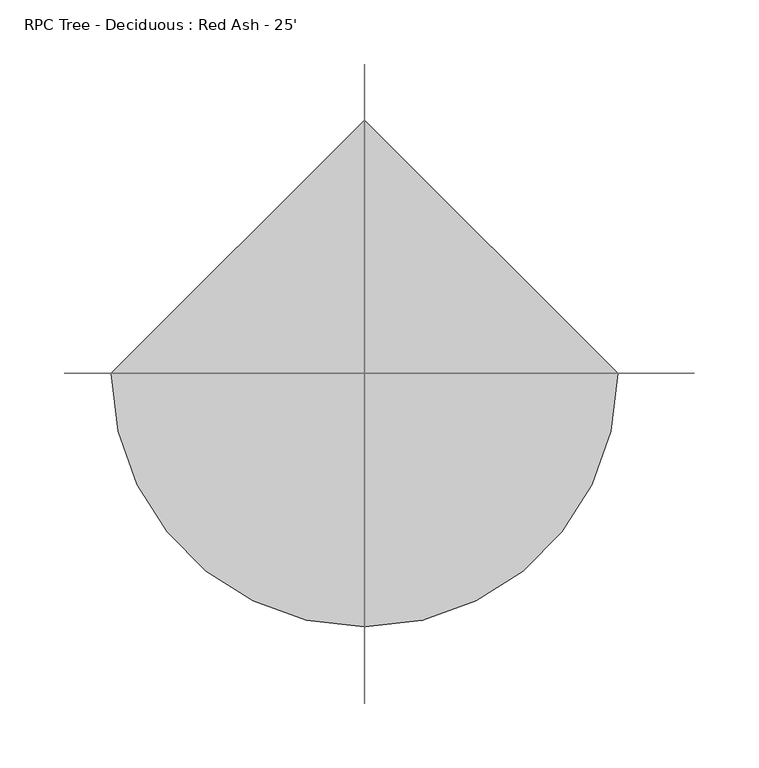
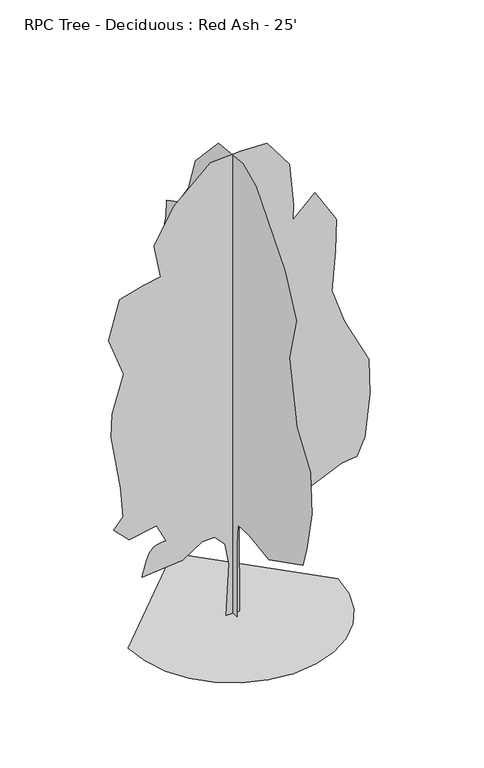
"""IFC4 building model written with IfcOpenShell, lengths in millimetres: geographic element geometry, RPC Tree - Deciduous : Red Ash - 25'."""

from ifc_helpers import new_model, si_unit, origin, place, context, project, spatial, triangles, source, transform, mapped, element, save


def rpc_tree_deciduous_red_ash_25_29d6c0be(model_context):
    return source(origin(), model_context, "Body", "Tessellation", [
        triangles([(-197.3943103, 0.0, 7.4e-06), (-192.1758061, -45.2297202, 7.4e-06), (-177.3137228, -86.7659884, 7.4e-06), (-153.9979766, -123.4187294, 7.4e-06), (-123.4187385, -153.9979948, 7.4e-06), (-86.7659612, -177.3136864, 7.4e-06), (-45.229702, -192.1758061, 7.4e-06), (8.6e-06, -197.3943103, 7.4e-06), (45.2297247, -192.1758243, 7.4e-06), (86.7659884, -177.3137228, 7.4e-06), (123.4187385, -153.9979766, 7.4e-06), (153.9980311, -123.4187385, 7.4e-06), (177.3137046, -86.7659612, 7.4e-06), (192.1758061, -45.2296929, 7.4e-06), (197.3943103, 1.73e-05, 7.4e-06), (-2.59e-05, 197.3943103, 7.4e-06), (-1.3e-06, -12.3415511, 0.0), (3e-06, -12.1496059, 143.3464828), (3.9e-06, -15.5858355, 184.536356), (1e-07, -52.659045, 186.979866), (-6.9e-06, -117.166958, 177.3968209), (-1.69e-05, -228.4431237, 233.8412498), (-1.7e-05, -241.3447163, 275.7714303), (-1.63e-05, -257.4717115, 353.1809132), (-1.34e-05, -252.6336529, 433.8158532), (-7e-06, -208.845846, 496.9220667), (-7e-07, -183.2878312, 619.2762262), (-4e-07, -205.8654139, 706.361899), (5.8e-06, -168.773401, 783.7714182), (1.88e-05, -75.2369229, 895.0476202), (2.38e-05, -32.784084, 914.1832981), (3.19e-05, 47.3281931, 906.3365387), (3.75e-05, 123.1250246, 825.701635), (3.78e-05, 145.7028252, 757.9682693), (3.99e-05, 179.5693627, 709.5872835), (4.32e-05, 216.6615754, 690.2349764), (4.24e-05, 218.2742676, 657.9809132), (4.23e-05, 227.9504757, 620.8889185), (3.93e-05, 211.8234986, 577.3460458), (3.96e-05, 226.3377653, 535.4159017), (3.93e-05, 240.8520501, 477.3587623), (3.85e-05, 237.6266656, 461.2317307), (3.45e-05, 210.2108063, 422.5269711), (3.28e-05, 208.4773911, 369.3079448), (3.16e-05, 206.9853855, 335.441262), (3.05e-05, 208.5980959, 293.511136), (2.89e-05, 210.2108245, 235.4540148), (2.61e-05, 187.6330238, 217.7142909), (2.17e-05, 145.7028797, 217.7142909), (2.19e-05, 165.0552595, 158.0444592), (2.06e-05, 161.8194105, 124.1861426), (1.82e-05, 132.363723, 147.3403706), (1.18e-05, 75.5355238, 132.8049115), (1.18e-05, 66.2054202, 162.8473093), (7.5e-06, 25.9095309, 162.4803077), (6e-06, 15.6961474, 147.4001417), (3.9e-06, 9.5459199, 98.1939791), (1.4e-06, 13.4599217, 1.5e-06), (-13.3045045, 6e-07, 5.4e-06), (-8.005377, -1.16e-05, 100.020203), (-15.5168751, -1.63e-05, 142.5532264), (-34.8945452, -1.8e-05, 163.8381281), (-58.0363739, -1.69e-05, 163.0435545), (-95.5521345, -1.24e-05, 138.6920794), (-171.3489706, -8.3e-06, 132.2413013), (-170.3004699, -8.8e-06, 136.411759), (-169.1814611, -9.4e-06, 140.72326), (-167.9214, -1e-05, 145.3168386), (-166.4497602, -1.06e-05, 150.3336381), (-164.6960155, -1.14e-05, 155.9145202), (-162.5896397, -1.22e-05, 162.2008008), (-160.0601066, -1.32e-05, 169.3333414), (-156.8723288, -1.41e-05, 175.948708), (-152.9228605, -1.49e-05, 180.7868029), (-148.3386563, -1.55e-05, 184.1437928), (-143.2466434, -1.59e-05, 186.3160621), (-137.7738306, -1.63e-05, 187.5995956), (-132.0470817, -1.67e-05, 188.2907417), (-126.1933965, -1.7e-05, 188.6857212), (-143.9330659, -2.04e-05, 224.1650781), (-195.5394453, -1.7e-05, 214.4888882), (-224.5679605, -1.92e-05, 243.5175124), (-206.8282911, -2.25e-05, 264.4825845), (-211.6663679, -2.92e-05, 322.5397239), (-229.4060555, -4.13e-05, 430.5904687), (-227.8176895, -4.67e-05, 475.3398448), (-206.3900911, -5.63e-05, 547.5990606), (-234.2441686, -6.42e-05, 624.1142303), (-213.279042, -7.39e-05, 698.2984377), (-169.736242, -7.74e-05, 711.1999758), (-136.6095848, -7.95e-05, 717.0435144), (-148.7711881, -8.67e-05, 782.1587259), (-111.6790935, -9.62e-05, 848.2793993), (-42.3330356, -0.0001068, 911.1746155), (14.1113616, -0.0001096, 914.4), (64.1050488, -0.0001116, 912.7872351), (106.0352065, -0.0001067, 856.3428606), (113.7446469, -9.72e-05, 773.7021927), (112.6376287, -9.35e-05, 743.396339), (154.4161378, -0.0001, 782.1587259), (194.7336079, -9.39e-05, 716.0380526), (193.1209156, -8.64e-05, 653.5811817), (185.9348898, -7.68e-05, 576.0782453), (209.2478927, -6.97e-05, 507.9999879), (255.811693, -6.08e-05, 416.3037681), (257.2962499, -5.26e-05, 347.1371324), (247.9526341, -4.24e-05, 264.4825481), (233.4383493, -3.77e-05, 230.6158653), (204.4097796, -3.6e-05, 227.3904808), (147.9653506, -3.05e-05, 201.5872956), (97.9716635, -2.41e-05, 166.1079387), (30.8971852, -2.46e-05, 194.9482568), (11.166104, -2.12e-05, 173.7161771), (12.4986284, -5e-07, 4.2e-06)], [[15, 16, 1], [14, 15, 1], [14, 1, 2], [13, 14, 2], [13, 2, 3], [13, 3, 4], [12, 13, 4], [11, 12, 4], [11, 4, 5], [11, 5, 6], [11, 6, 7], [11, 7, 8], [11, 8, 9], [11, 9, 10], [50, 51, 52], [57, 58, 17], [57, 17, 18], [56, 57, 18], [56, 18, 19], [55, 56, 19], [49, 50, 52], [52, 53, 54], [49, 52, 54], [35, 36, 37], [46, 47, 48], [46, 48, 49], [21, 22, 23], [20, 21, 23], [20, 23, 24], [20, 24, 25], [20, 25, 26], [19, 20, 26], [19, 26, 27], [45, 46, 49], [31, 32, 33], [30, 31, 33], [29, 30, 33], [29, 33, 34], [28, 29, 34], [27, 28, 34], [19, 27, 34], [19, 34, 35], [19, 35, 37], [19, 37, 38], [19, 38, 39], [19, 39, 40], [19, 40, 41], [19, 41, 42], [19, 42, 43], [19, 43, 44], [19, 44, 45], [19, 45, 49], [19, 49, 54], [55, 19, 54], [64, 65, 66], [64, 66, 67], [64, 67, 68], [99, 100, 101], [64, 68, 69], [64, 69, 70], [64, 70, 71], [114, 59, 60], [113, 114, 60], [113, 60, 61], [113, 61, 62], [64, 71, 72], [64, 72, 73], [64, 73, 74], [64, 74, 75], [64, 75, 76], [64, 76, 77], [64, 77, 78], [64, 78, 79], [63, 64, 79], [81, 82, 83], [80, 81, 83], [99, 101, 102], [107, 108, 109], [110, 111, 112], [88, 89, 90], [87, 88, 90], [87, 90, 91], [80, 83, 84], [95, 96, 97], [95, 97, 98], [94, 95, 98], [93, 94, 98], [92, 93, 98], [91, 92, 98], [91, 98, 99], [87, 91, 99], [87, 99, 102], [87, 102, 103], [87, 103, 104], [86, 87, 104], [85, 86, 104], [84, 85, 104], [80, 84, 104], [80, 104, 105], [80, 105, 106], [80, 106, 107], [80, 107, 109], [80, 109, 110], [80, 110, 112], [79, 80, 112], [63, 79, 112], [62, 63, 112], [113, 62, 112]], closed=False),
    ])


if __name__ == "__main__":
    model = new_model("IFC4")
    model_context = context("Model", 3, world=origin())
    ifc_project = project(units=[si_unit("LENGTHUNIT", "METRE", prefix="MILLI")], contexts=[model_context])
    site = spatial("IfcSite", under=ifc_project)
    building = spatial("IfcBuilding", under=site)
    placement = place(None, origin())
    rpc_tree_deciduous_red_ash_25_shape = rpc_tree_deciduous_red_ash_25_29d6c0be(model_context)
    element("IfcGeographicElement", 1, ObjectType="RPC Tree - Deciduous : Red Ash - 25'", at=placement, inside=building, context=model_context, shape_type="MappedRepresentation", body=[
        mapped(rpc_tree_deciduous_red_ash_25_shape, transform((0.0, 0.0, 0.0), x_axis=(1.0, 0.0, 0.0), y_axis=(0.0, 1.0, 0.0), z_axis=(0.0, 0.0, 1.0))),
    ])
    save(model, "model.ifc")

# Revit data of these elements
# Type "RPC Tree - Deciduous : Red Ash - 25'"
#   built-in parameter 1005198 = "{2, 15},{22, RPC-8-G3GR-497X-PHW5-6},{1, 0},{1, 0},{2, 15},{1, 8},{5, Color},{1, 0},{1, 0},{3, 0.8},{3, 0.8},{3, 0.8},{1, 8},{7, BBoxMin},{1, 0},{1, 0},{1, 0},{1, 0},{1, 0},{1, 8},{7, BBoxMax},{1, 0},{1, 0},{1, 0},{1, 0},{1, 0},{2, 11},{9, RPCTypeId},{1, 0},{1, 0},{22, RPC-8-G3GR-497X-PHW5-6},{1, 6},{14, RPCPlantHeight},{1, 0},{1, 0},{2, 25},{2, 11},{7, keyword},{1, 0},{1, 0},{34, :RPCs:Trees [General]:Geometry:RPC},{2, 11},{8, category},{1, 0},{1, 0},{15, Trees [General]},{2, 11},{12, LocalizedUID},{1, 0},{1, 0},{7, Red Ash},{2, 14},{6, Height},{1, 0},{1, 0},{2, 25},{1, 2},{16, Cast Reflections},{1, 0},{1, 0},{1, 0},{1, 2},{6, Jitter},{1, 0},{1, 0},{1, 1},{1, 2},{9, Billboard},{1, 0},{1, 0},{1, 0},{1, 2},{12, Cast Shadows},{1, 0},{1, 0},{1, 1},{1, 2},{20, Apply Filter Effects},{1, 0},{1, 0},{1, 0},{2, 11},{28, Apply Filter Effects-Text-FC},{1, 0},{1, 0},{4, None},{21, assetlibrary_base.fbx},{1, 5},"
#   built-in parameter 1005195 = "RPC-8-G3GR-497X-PHW5-6"
#   Type Comments = "Red Maple"
#   Assembly Code = "G2050500"
#   Height = 3' - 0"
#   Default Elevation = 0
